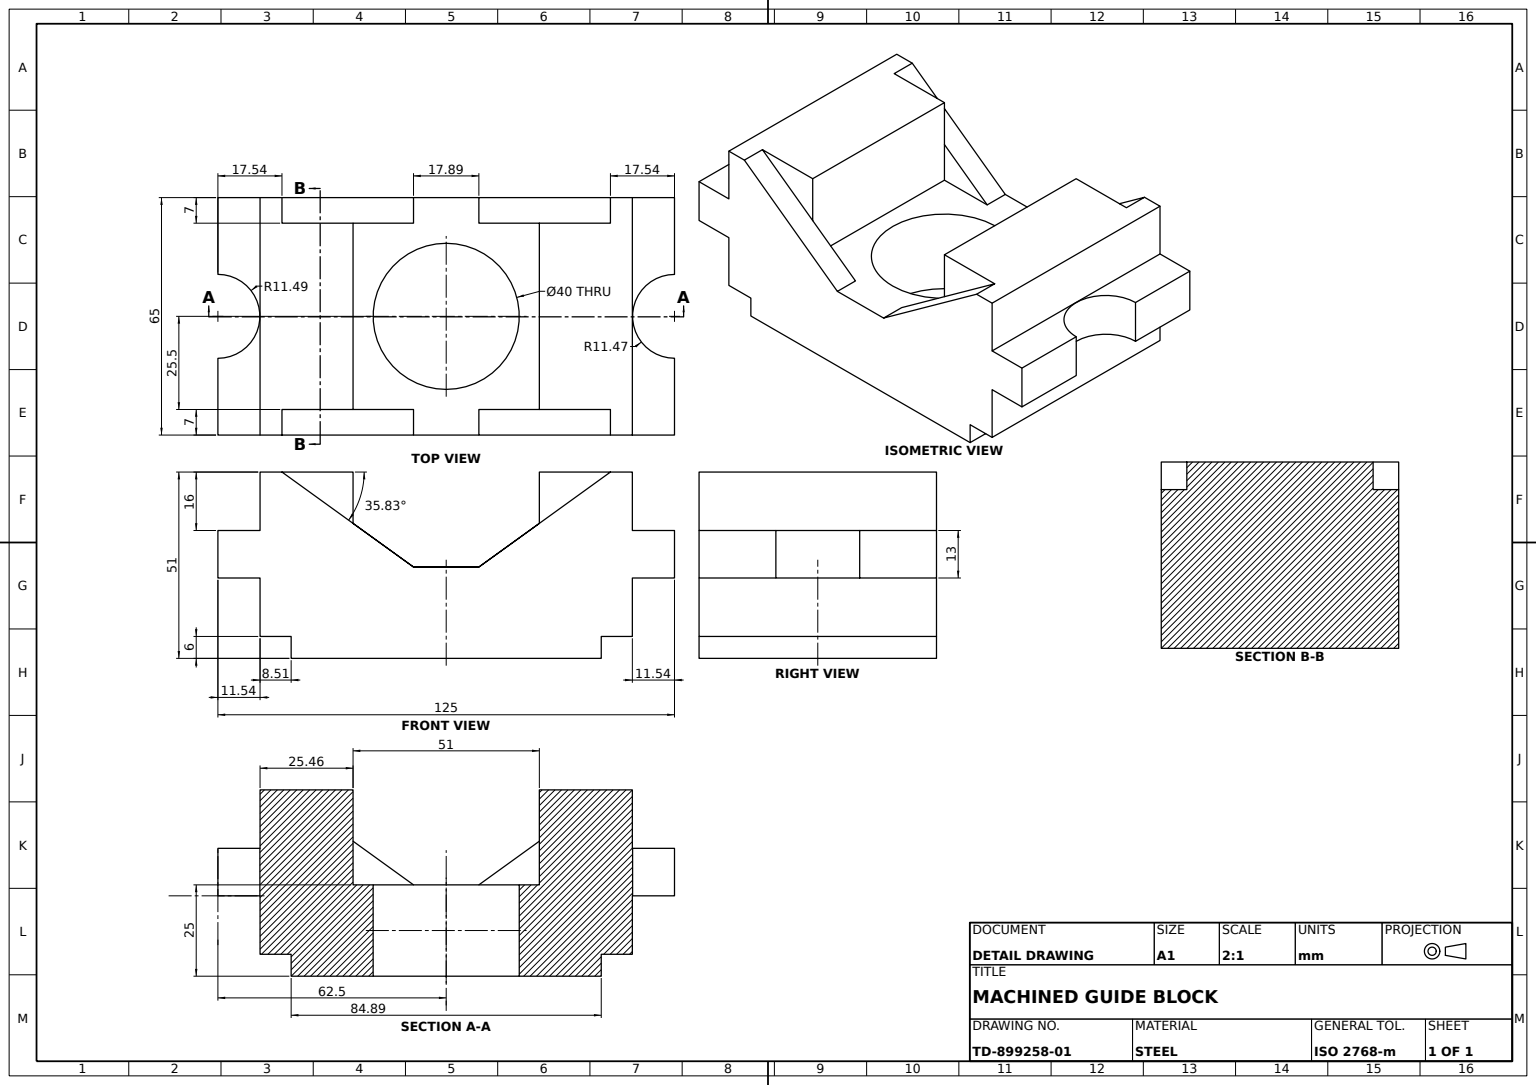
from build123d import *

# Parameters (mm, degrees)
STEPPED_CRADLE_BLOCK_65_DEPTH = 65
RAISED_BOSS_SKETCH_W          = 19.460384675
RAISED_BOSS_SKETCH_H          = 51
RAISED_BOSS_DEPTH             = 26
CRADLE_SLOT_SKETCH_W          = 51
CRADLE_SLOT_SKETCH_H          = 51
CRADLE_SLOT_CUT_DEPTH         = 41
CENTER_HOLE_SKETCH_R          = 20
CENTER_HOLE_40_DEPTH          = 41
FRONT_RELIEF_SKETCH_R         = 11.472679984
FRONT_RELIEF_SKETCH_R_2       = 11.491831568
FRONT_RELIEF_CUT_DEPTH        = 41


with BuildPart() as part:
    # Stepped Cradle Profile Sketch → Stepped Cradle Block 65 (new body)
    with BuildSketch(Plane.XY):
        Polygon((-42.445795816, 0), (-42.445795816, 6), (-50.960384675, 6), (-50.960384675, 22), (-62.5, 22), (-62.5, 35), (-50.960384675, 35), (-50.960384675, 51), (-44.960384675, 51), (-8.945795816, 25), (8.945795816, 25), (44.960384675, 51), (50.960384675, 51), (50.960384675, 35), (62.5, 35), (62.5, 22), (50.960384675, 22), (50.960384675, 6), (42.445795816, 6), (42.445795816, 0), (8.945795816, 0), (-8.945795816, 0), align=None)
    extrude(amount=-STEPPED_CRADLE_BLOCK_65_DEPTH)

    # Raised Boss Sketch → Raised Boss (add)
    with BuildSketch(Plane(origin=(0, 25, 0), x_dir=(1, 0, 0), z_dir=(0, 1, 0))):
        with Locations((-35.230192338, 32.5)):
            Rectangle(RAISED_BOSS_SKETCH_W, RAISED_BOSS_SKETCH_H)
        with Locations((35.230192338, 32.5)):
            Rectangle(RAISED_BOSS_SKETCH_W, RAISED_BOSS_SKETCH_H)
    extrude(amount=RAISED_BOSS_DEPTH)

    # Cradle Slot Sketch → Cradle Slot Cut (cut)
    with BuildSketch(Plane(origin=(0, 25, 0), x_dir=(1, 0, 0), z_dir=(0, 1, 0))):
        with Locations((0, 32.5)):
            Rectangle(CRADLE_SLOT_SKETCH_W, CRADLE_SLOT_SKETCH_H)
    extrude(amount=CRADLE_SLOT_CUT_DEPTH, mode=Mode.SUBTRACT)

    # Center Hole Sketch → Center Hole Ø40 (cut)
    with BuildSketch(Plane(origin=(0, 25, 0), x_dir=(1, 0, 0), z_dir=(0, 1, 0))):
        with Locations(Location((0, 32.5, 0), (0, 0, 270))):
            Circle(CENTER_HOLE_SKETCH_R)
    extrude(amount=-CENTER_HOLE_40_DEPTH, mode=Mode.SUBTRACT)

    # Front Relief Sketch → Front Relief Cut (cut)
    with BuildSketch(Plane(origin=(0, 35, 0), x_dir=(1, 0, 0), z_dir=(0, 1, 0))):
        with Locations((62.5, 32.5)):
            Circle(FRONT_RELIEF_SKETCH_R)
        with Locations((-62.5, 32.5)):
            Circle(FRONT_RELIEF_SKETCH_R_2)
    extrude(amount=-FRONT_RELIEF_CUT_DEPTH, mode=Mode.SUBTRACT)


solid = part.part
